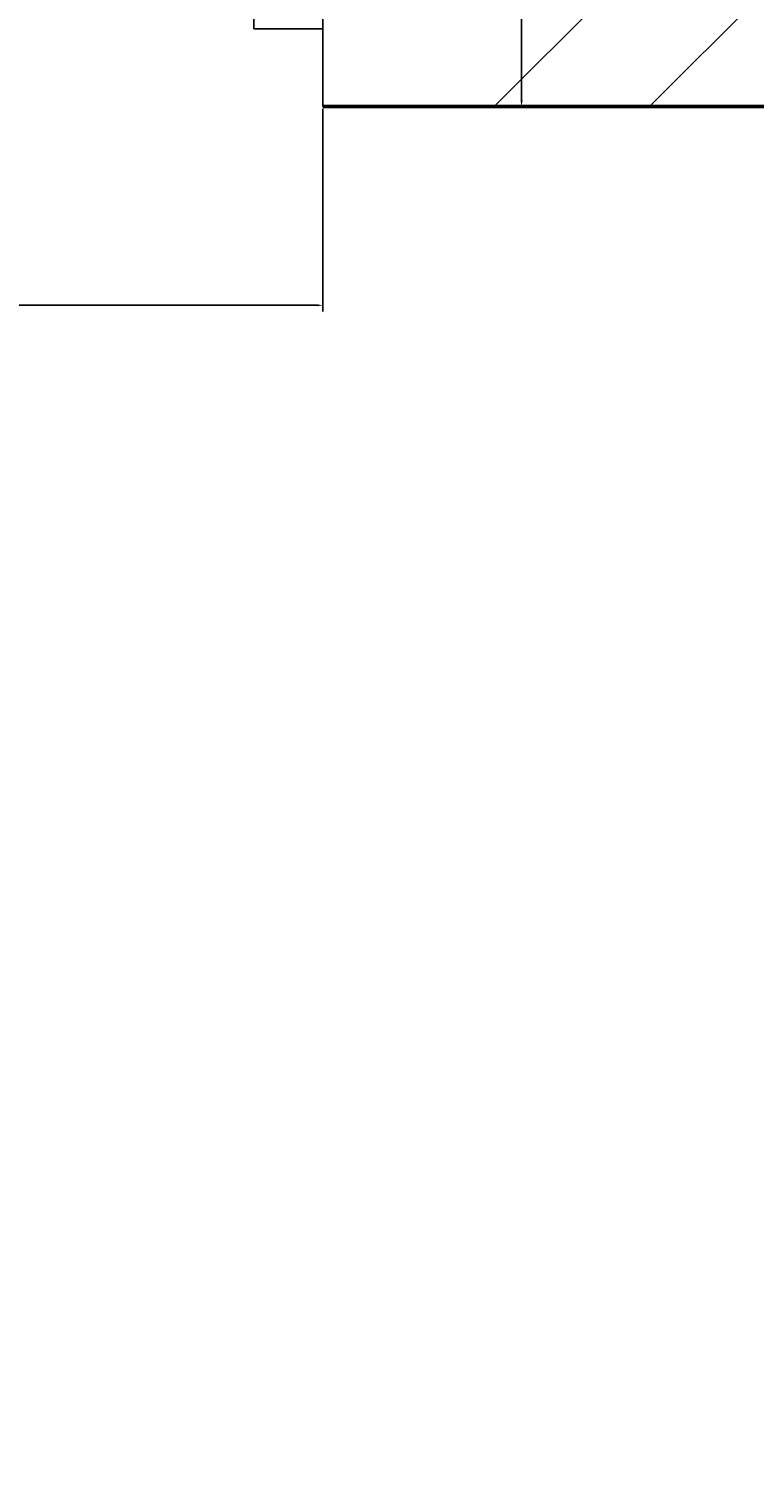
# Model space of a CAD drawing. Units: inches. Extents: x 963 to 2075, y 289 to 2657.
# Tile 65 of 98: x 1245 to 1266, y 2284 to 2325. Entities that reach past the tile are written whole.
import ezdxf

# ---------------------------------------------------------------- set-up
doc = ezdxf.new("R2010")
doc.units = ezdxf.units.IN
for name, color, linetype, lineweight in [('A-ANNO-DIMS', 2, 'Continuous', 18), ('A-DOOR', 4, 'Continuous', 25), ('A-WALL', 7, 'Continuous', 50), ('A-WALL-PATT', 8, 'Continuous', 13)]:
    doc.layers.add(name, color=color, linetype=linetype, lineweight=lineweight)
doc.styles.get("Standard").update_dxf_attribs({"font": 'arial.ttf'})
doc.dimstyles.get("Standard").update_dxf_attribs({"dimtxt": 0.18, "dimasz": 0.18, "dimexe": 0.18, "dimexo": 0.0625, "dimgap": 0.09, "dimtad": 0, "dimtih": 1, "dimtoh": 1, "dimdec": 4, "dimzin": 0, "dimdsep": 46, "dimtxsty": 'Standard', "dimcen": 0.09, "dimadec": 0, "dimazin": 0, "dimtfac": 1, "dimtdec": 4, "dimtofl": 0, "dimtmove": 0, "dimatfit": 3, "dimfxl": 1, "dimtolj": 1, "dimtzin": 0, "dimarcsym": 0})

# ---------------------------------------------------------------- blocks, each defined once
blk = doc.blocks.new('DOOR-1')
for p, q in [((25.385, 2.25), (25.385, 38.25)), ((0.325, 4.5), (0.325, 0)), ((27.385, 4.5), (27.385, 0)), ((0.325, 0), (0.325, 2.25)), ((0.325, 2.25), (2.325, 2.25)), ((27.385, 2.25), (25.385, 2.25)), ((27.385, 0), (27.385, 2.25))]:
    blk.add_line(p, q)
blk.add_arc((25.385, 12.864), 25.386, 90, 204.7158)
blk = doc.blocks.new('*D30')
at = {"layer": 'A-ANNO-DIMS', "color": 0, "lineweight": -2, "transparency": 16777216}
for p, q in [((1253.776, 2361.068), (1259.631, 2361.068)), ((1259.451, 2360.888), (1259.451, 2342.126)), ((1259.451, 2322.998), (1259.451, 2341.759)), ((1253.776, 2322.818), (1259.631, 2322.818))]:
    blk.add_line(p, q, dxfattribs=at)
at = {"layer": 'A-ANNO-DIMS', "color": 0, "transparency": 16777216}
for points in [[(1259.421, 2360.888), (1259.481, 2360.888), (1259.451, 2361.068)], [(1259.421, 2322.998), (1259.481, 2322.998), (1259.451, 2322.818)]]:
    blk.add_solid(points, dxfattribs=at)
at = {"layer": 'Defpoints', "color": 0, "transparency": 16777216}
for p in [(1253.714, 2361.068), (1259.451, 2361.068), (1253.714, 2322.818)]:
    blk.add_point(p, dxfattribs=at)
at = {"layer": 'A-ANNO-DIMS', "color": 0, "transparency": 16777216, "insert": (1259.451, 2341.943), "char_height": 0.18, "attachment_point": 5}
blk.add_mtext('\\A1;DOOR D1 38 TYP.', dxfattribs=at)
blk = doc.blocks.new('*D31')
at = {"layer": 'A-ANNO-DIMS', "color": 0, "lineweight": -2, "transparency": 16777216}
for p, q in [((1225.036, 2322.755), (1225.036, 2316.9)), ((1253.714, 2322.755), (1253.714, 2316.9)), ((1225.216, 2317.08), (1238.845, 2317.08)), ((1253.534, 2317.08), (1239.904, 2317.08))]:
    blk.add_line(p, q, dxfattribs=at)
at = {"layer": 'A-ANNO-DIMS', "color": 0, "transparency": 16777216}
for points in [[(1225.216, 2317.11), (1225.216, 2317.05), (1225.036, 2317.08)], [(1253.534, 2317.11), (1253.534, 2317.05), (1253.714, 2317.08)]]:
    blk.add_solid(points, dxfattribs=at)
at = {"layer": 'Defpoints', "color": 0, "transparency": 16777216}
for p in [(1225.036, 2322.818), (1253.714, 2322.818), (1253.714, 2317.08)]:
    blk.add_point(p, dxfattribs=at)
at = {"layer": 'A-ANNO-DIMS', "color": 0, "transparency": 16777216, "insert": (1239.375, 2317.08), "char_height": 0.18, "attachment_point": 5}
blk.add_mtext('\\A1;29 TYP.', dxfattribs=at)

msp = doc.modelspace()

# ---------------------------------------------------------------- hatches: boundary and pattern name
at = {"layer": 'A-WALL-PATT'}
h = msp.add_hatch(dxfattribs=at)
h.set_pattern_fill('ANSI32', color=256)
h.paths.add_polyline_path([(1296.922, 2558.318), (1203.922, 2558.318), (1203.922, 2493.818), (1191.533, 2493.818), (1191.533, 2489.318), (1211.063, 2489.318), (1211.063, 2492.02), (1211.063, 2493.818), (1208.422, 2493.818), (1208.422, 2553.818), (1292.422, 2553.818), (1292.422, 2538.863), (1296.922, 2538.863)])
h.paths.add_polyline_path([(1442.422, 2558.318), (1349.422, 2558.318), (1349.422, 2538.943), (1353.922, 2538.943), (1353.922, 2553.818), (1437.922, 2553.818), (1437.922, 2493.818), (1434.542, 2493.818), (1434.542, 2489.318), (1448.311, 2489.318), (1448.311, 2491.568), (1448.311, 2493.818), (1442.422, 2493.818)])
h.paths.add_polyline_path([(1415.554, 2491.568), (1415.554, 2493.818), (1340.941, 2493.818), (1340.941, 2489.318), (1371.922, 2489.318), (1371.922, 2378.318), (1367.596, 2378.318), (1367.596, 2373.818), (1371.922, 2373.818), (1371.922, 2355.185), (1376.422, 2355.185), (1376.422, 2489.318), (1415.554, 2489.318)])
h.paths.add_polyline_path([(1304.941, 2491.568), (1304.941, 2493.818), (1296.922, 2493.818), (1296.922, 2514.863), (1292.422, 2514.863), (1292.422, 2493.818), (1232.808, 2493.818), (1232.808, 2489.318), (1256.422, 2489.318), (1256.422, 2327.318), (1253.714, 2327.318), (1253.714, 2322.818), (1328.422, 2322.818), (1328.422, 2331.147), (1323.922, 2331.147), (1323.922, 2327.318), (1260.922, 2327.318), (1260.922, 2373.818), (1323.922, 2373.818), (1323.922, 2357.812), (1328.422, 2357.812), (1328.422, 2373.818), (1346.007, 2373.818), (1346.007, 2376.068), (1346.007, 2378.318), (1260.922, 2378.318), (1260.922, 2489.318), (1304.941, 2489.318)])
h.paths.add_polyline_path([(1226.654, 2327.318), (1124.422, 2327.318), (1124.422, 2347.447), (1119.922, 2347.447), (1119.922, 2322.818), (1163.422, 2322.818), (1163.422, 2305.435), (1165.672, 2305.435), (1167.922, 2305.435), (1167.922, 2322.818), (1226.654, 2322.818), (1226.654, 2325.068)])
h.paths.add_polyline_path([(1095.922, 2489.318), (1124.422, 2489.318), (1131.533, 2489.318), (1131.533, 2491.568), (1131.533, 2493.818), (1119.922, 2493.818), (1091.422, 2493.818), (1091.422, 2417.318), (1095.922, 2417.318), (1119.922, 2417.318), (1119.922, 2407.447), (1124.422, 2407.447), (1124.422, 2421.818), (1095.922, 2421.818)])
h.paths.add_polyline_path([(1512.922, 2558.318), (1508.422, 2558.318), (1508.422, 2493.818), (1503.401, 2493.818), (1503.401, 2489.318), (1508.422, 2489.318), (1508.422, 2327.318), (1376.422, 2327.318), (1376.422, 2330.273), (1371.922, 2330.273), (1371.922, 2298.744), (1376.422, 2298.744), (1376.422, 2322.818), (1508.422, 2322.818), (1508.422, 2165.318), (1504.255, 2165.318), (1504.255, 2160.818), (1508.422, 2160.818), (1508.422, 2108.318), (1512.922, 2108.318), (1512.922, 2160.818), (1516.182, 2160.818), (1516.182, 2163.068), (1516.182, 2165.318), (1512.922, 2165.318), (1512.922, 2322.818), (1644.922, 2322.818), (1644.922, 2298.744), (1649.422, 2298.744), (1649.422, 2322.818), (1649.422, 2330.944), (1647.172, 2330.944), (1644.922, 2330.944), (1644.922, 2327.318), (1512.922, 2327.318), (1512.922, 2489.318), (1516.759, 2489.318), (1516.759, 2491.568), (1516.759, 2493.818), (1512.922, 2493.818)])
h.paths.add_polyline_path([(1671.922, 2558.318), (1578.922, 2558.318), (1578.922, 2493.818), (1573.526, 2493.818), (1573.526, 2489.318), (1586.537, 2489.318), (1586.537, 2491.568), (1586.537, 2493.818), (1583.422, 2493.818), (1583.422, 2553.818), (1667.422, 2553.818), (1667.422, 2541.109), (1671.922, 2541.109)])
h.paths.add_polyline_path([(1681.257, 2493.818), (1671.922, 2493.818), (1671.922, 2517.109), (1667.422, 2517.109), (1667.422, 2493.818), (1610.218, 2493.818), (1610.218, 2489.318), (1644.922, 2489.318), (1644.922, 2357.865), (1649.422, 2357.865), (1649.422, 2373.818), (1652.203, 2373.818), (1652.203, 2375.827), (1652.203, 2378.318), (1649.422, 2378.318), (1649.422, 2489.318), (1681.257, 2489.318), (1681.257, 2491.568)])
h.paths.add_polyline_path([(1821.922, 2558.318), (1728.922, 2558.318), (1728.922, 2541), (1733.422, 2541), (1733.422, 2553.818), (1817.422, 2553.818), (1817.422, 2493.818), (1813.507, 2493.818), (1813.507, 2489.318), (1830.078, 2489.318), (1830.078, 2491.568), (1830.078, 2493.818), (1821.922, 2493.818)])
h.paths.add_polyline_path([(1794.244, 2493.818), (1717.257, 2493.818), (1717.257, 2489.318), (1760.422, 2489.318), (1760.422, 2378.318), (1674.401, 2378.318), (1674.401, 2373.818), (1692.922, 2373.818), (1692.922, 2356.954), (1697.422, 2356.954), (1697.422, 2373.818), (1760.422, 2373.818), (1760.422, 2327.318), (1697.422, 2327.318), (1697.422, 2333.341), (1692.922, 2333.341), (1692.922, 2322.818), (1768.037, 2322.818), (1768.037, 2325.068), (1768.037, 2327.318), (1764.922, 2327.318), (1764.922, 2489.318), (1794.244, 2489.318)])
h.paths.add_polyline_path([(1733.422, 2517), (1728.922, 2517), (1728.922, 2493.818), (1733.422, 2493.818)], flags=17)
h.paths.add_polyline_path([(1929.922, 2493.818), (1890.078, 2493.818), (1890.078, 2489.318), (1896.922, 2489.318), (1925.422, 2489.318), (1925.422, 2421.818), (1896.922, 2421.818), (1896.922, 2408.318), (1901.422, 2408.318), (1901.422, 2417.318), (1925.422, 2417.318), (1929.922, 2417.318)])
h.paths.add_polyline_path([(1901.422, 2348.318), (1896.922, 2348.318), (1896.922, 2327.318), (1800.423, 2327.318), (1800.423, 2322.818), (1853.422, 2322.818), (1853.422, 2309.453), (1857.922, 2309.453), (1857.922, 2322.818), (1901.422, 2322.818)])
h.paths.add_polyline_path([(1857.922, 2249.453), (1853.422, 2249.453), (1853.422, 2214.818), (1686.309, 2214.818), (1686.309, 2210.318), (1853.422, 2210.318), (1853.422, 2202.134), (1857.922, 2202.134), (1857.922, 2210.318)])
h.paths.add_polyline_path([(1857.922, 2142.134), (1853.422, 2142.134), (1853.422, 2115.422), (1841.422, 2115.422), (1841.422, 2088.531), (1841.422, 2046.949), (1845.922, 2046.949), (1845.922, 2110.922), (1905.922, 2110.922), (1905.922, 2092.517), (1910.422, 2092.517), (1910.422, 2115.422), (1857.922, 2115.422)])
h.paths.add_polyline_path([(1532.436, 1482.342), (1573.456, 1482.342), (1573.456, 1501), (1532.436, 1501)], flags=9)
h.paths.add_polyline_path([(1438.658, 1486.302), (1479.678, 1486.302), (1479.678, 1504.96), (1438.658, 1504.96)], flags=9)
h.paths.add_polyline_path([(1411.215, 1365.308), (1659.139, 1365.308), (1659.139, 1402.401), (1411.215, 1402.401)], flags=9)
h.paths.add_polyline_path([(1185.671, 2296.298), (1248.16, 2296.298), (1248.16, 2314.955), (1185.671, 2314.955)], flags=9)
h.paths.add_polyline_path([(1177.31, 2187.35), (1216.15, 2187.35), (1216.15, 2206.007), (1177.31, 2206.007)], flags=9)
h.paths.add_polyline_path([(1295.101, 1602.083), (1328.26, 1602.083), (1328.26, 1620.741), (1295.101, 1620.741)], flags=9)
h.paths.add_polyline_path([(1525.126, 2005.99), (1558.39, 2005.99), (1558.39, 2024.648), (1525.126, 2024.648)], flags=9)
h.paths.add_polyline_path([(1459.606, 1977.125), (1472.195, 1977.125), (1472.195, 1987.429), (1459.606, 1987.429)], flags=9)
h.paths.add_polyline_path([(1467.815, 2053.676), (1480.018, 2053.676), (1480.018, 2063.979), (1467.815, 2063.979)], flags=9)
h.paths.add_polyline_path([(1555.184, 2119.02), (1584.563, 2119.02), (1584.563, 2137.678), (1555.184, 2137.678)], flags=25)
h.paths.add_polyline_path([(1405.389, 2115.291), (1444.478, 2115.291), (1444.478, 2133.948), (1405.389, 2133.948)], flags=25)
h.paths.add_polyline_path([(1698.482, 2004.259), (1727.695, 2004.259), (1727.695, 2022.916), (1698.482, 2022.916)], flags=9)
h.paths.add_polyline_path([(1612.158, 1972.855), (1629.016, 1972.855), (1629.016, 1983.159), (1612.158, 1983.159)], flags=9)
h.paths.add_polyline_path([(1608.289, 2060.036), (1625.147, 2060.036), (1625.147, 2070.34), (1608.289, 2070.34)], flags=9)
h.paths.add_polyline_path([(1527.954, 1684.402), (1566.795, 1684.402), (1566.795, 1703.06), (1527.954, 1703.06)], flags=9)
h.paths.add_polyline_path([(1422.792, 1683.59), (1461.633, 1683.59), (1461.633, 1702.247), (1422.792, 1702.247)], flags=9)
h.paths.add_polyline_path([(1531.262, 1732.459), (1574.015, 1732.459), (1574.015, 1751.116), (1531.262, 1751.116)], flags=9)
h.paths.add_polyline_path([(1402.872, 1732.845), (1439.799, 1732.845), (1439.799, 1751.502), (1402.872, 1751.502)], flags=9)
h.paths.add_polyline_path([(1243.122, 1923.132), (1281.962, 1923.132), (1281.962, 1941.79), (1243.122, 1941.79)], flags=9)
h.paths.add_polyline_path([(1181.752, 1792.268), (1244.241, 1792.268), (1244.241, 1810.926), (1181.752, 1810.926)], flags=9)
h.paths.add_polyline_path([(1265.822, 1670.3), (1316.071, 1670.3), (1316.071, 1688.957), (1265.822, 1688.957)], flags=9)
h.paths.add_polyline_path([(1140.263, 1676.054), (1179.104, 1676.054), (1179.104, 1694.711), (1140.263, 1694.711)], flags=9)
h.paths.add_polyline_path([(1107.49, 1490.889), (1143.374, 1490.889), (1143.374, 1509.546), (1107.49, 1509.546)], flags=9)
h.paths.add_polyline_path([(1217.584, 1483.899), (1246.741, 1483.899), (1246.741, 1502.556), (1217.584, 1502.556)], flags=9)
h.paths.add_polyline_path([(1389.21, 1486.919), (1418.367, 1486.919), (1418.367, 1505.576), (1389.21, 1505.576)], flags=9)
h.paths.add_polyline_path([(1672.208, 1602.083), (1705.366, 1602.083), (1705.366, 1620.741), (1672.208, 1620.741)], flags=9)
h.paths.add_polyline_path([(1752.082, 1522.638), (1781.24, 1522.638), (1781.24, 1541.295), (1752.082, 1541.295)], flags=9)
h.paths.add_polyline_path([(1848.275, 1491.26), (1884.158, 1491.26), (1884.158, 1509.918), (1848.275, 1509.918)], flags=9)
h.paths.add_polyline_path([(1822.47, 1685.62), (1861.31, 1685.62), (1861.31, 1704.278), (1822.47, 1704.278)], flags=9)
h.paths.add_polyline_path([(1713.195, 1672.232), (1763.444, 1672.232), (1763.444, 1690.889), (1713.195, 1690.889)], flags=9)
h.paths.add_polyline_path([(1736.619, 1790.578), (1799.109, 1790.578), (1799.109, 1809.235), (1736.619, 1809.235)], flags=9)
h.paths.add_polyline_path([(1691.491, 1916.355), (1730.332, 1916.355), (1730.332, 1935.013), (1691.491, 1935.013)], flags=9)
h.paths.add_polyline_path([(1764.872, 1973.922), (1794.306, 1973.922), (1794.306, 1992.58), (1764.872, 1992.58)], flags=9)
h.paths.add_polyline_path([(1767.854, 2034.017), (1797.288, 2034.017), (1797.288, 2052.674), (1767.854, 2052.674)], flags=9)
h.paths.add_polyline_path([(1851.593, 2060.331), (1880.751, 2060.331), (1880.751, 2078.989), (1851.593, 2078.989)], flags=25)
h.paths.add_polyline_path([(1688.491, 2086.874), (1727.332, 2086.874), (1727.332, 2105.531), (1688.491, 2105.531)], flags=9)
h.paths.add_polyline_path([(1537.743, 2293.581), (1580.495, 2293.581), (1580.495, 2312.239), (1537.743, 2312.239)], flags=25)
h.paths.add_polyline_path([(1425.587, 2296.109), (1468.34, 2296.109), (1468.34, 2314.766), (1425.587, 2314.766)], flags=25)
h.paths.add_polyline_path([(1278.518, 2004.184), (1307.72, 2004.184), (1307.72, 2022.841), (1278.518, 2022.841)], flags=9)
h.paths.add_polyline_path([(1193.282, 1973.635), (1222.715, 1973.635), (1222.715, 1992.292), (1193.282, 1992.292)], flags=9)
h.paths.add_polyline_path([(1192.411, 2040.577), (1221.845, 2040.577), (1221.845, 2059.234), (1192.411, 2059.234)], flags=9)
h.paths.add_polyline_path([(1130.603, 1951.393), (1159.76, 1951.393), (1159.76, 1970.05), (1130.603, 1970.05)], flags=9)
h.paths.add_polyline_path([(1132.827, 2052.494), (1161.984, 2052.494), (1161.984, 2071.151), (1132.827, 2071.151)], flags=9)
h.paths.add_polyline_path([(1265.128, 2334.619), (1315.377, 2334.619), (1315.377, 2353.277), (1265.128, 2353.277)], flags=25)
h.paths.add_polyline_path([(1136.741, 2330.785), (1175.582, 2330.785), (1175.582, 2349.443), (1136.741, 2349.443)], flags=9)
h.paths.add_polyline_path([(1287.422, 2417.204), (1320.58, 2417.204), (1320.58, 2435.861), (1287.422, 2435.861)], flags=25)
h.paths.add_polyline_path([(1430.988, 2329.159), (1469.828, 2329.159), (1469.828, 2347.816), (1430.988, 2347.816)], flags=25)
h.paths.add_polyline_path([(1525.424, 2329.213), (1564.264, 2329.213), (1564.264, 2347.87), (1525.424, 2347.87)], flags=25)
h.paths.add_polyline_path([(1684.525, 2382.799), (1717.683, 2382.799), (1717.683, 2401.457), (1684.525, 2401.457)], flags=25)
h.paths.add_polyline_path([(1704.805, 2340.293), (1755.054, 2340.293), (1755.054, 2358.95), (1704.805, 2358.95)], flags=25)
h.paths.add_polyline_path([(1694.113, 2287.757), (1756.602, 2287.757), (1756.602, 2306.414), (1694.113, 2306.414)], flags=9)
h.paths.add_polyline_path([(1815.778, 2329.861), (1854.618, 2329.861), (1854.618, 2348.518), (1815.778, 2348.518)], flags=9)
h.paths.add_polyline_path([(1842.873, 2514.256), (1878.756, 2514.256), (1878.756, 2532.914), (1842.873, 2532.914)], flags=9)
h.paths.add_polyline_path([(1769.513, 2531.447), (1798.671, 2531.447), (1798.671, 2550.104), (1769.513, 2550.104)], flags=25)
h.paths.add_polyline_path([(1594.772, 2518.468), (1623.93, 2518.468), (1623.93, 2537.125), (1594.772, 2537.125)], flags=25)
h.paths.add_polyline_path([(1520.723, 2516.185), (1556.606, 2516.185), (1556.606, 2534.842), (1520.723, 2534.842)], flags=25)
h.paths.add_polyline_path([(1464.456, 2516.694), (1500.34, 2516.694), (1500.34, 2535.351), (1464.456, 2535.351)], flags=25)
h.paths.add_polyline_path([(1365.696, 2528.97), (1394.854, 2528.97), (1394.854, 2547.627), (1365.696, 2547.627)], flags=25)
h.paths.add_polyline_path([(1222.838, 2516.231), (1251.995, 2516.231), (1251.995, 2534.889), (1222.838, 2534.889)], flags=25)
h.paths.add_polyline_path([(1104.545, 2509.6), (1140.429, 2509.6), (1140.429, 2528.257), (1104.545, 2528.257)], flags=9)
h = msp.add_hatch(dxfattribs=at)
h.set_pattern_fill('ANSI32', color=256)
h.paths.add_polyline_path([(1335.968, 2212.568), (1335.968, 2214.818), (1167.922, 2214.818), (1167.922, 2245.435), (1163.422, 2245.435), (1163.422, 2210.318), (1163.422, 2194.812), (1167.922, 2194.812), (1167.922, 2210.318), (1335.968, 2210.318)])
h.paths.add_polyline_path([(1532.436, 1482.342), (1573.456, 1482.342), (1573.456, 1501), (1532.436, 1501)], flags=9)
h.paths.add_polyline_path([(1438.658, 1486.302), (1479.678, 1486.302), (1479.678, 1504.96), (1438.658, 1504.96)], flags=9)
h.paths.add_polyline_path([(1411.215, 1365.308), (1659.139, 1365.308), (1659.139, 1402.401), (1411.215, 1402.401)], flags=9)
h.paths.add_polyline_path([(1185.671, 2296.298), (1248.16, 2296.298), (1248.16, 2314.955), (1185.671, 2314.955)], flags=9)
h.paths.add_polyline_path([(1177.31, 2187.35), (1216.15, 2187.35), (1216.15, 2206.007), (1177.31, 2206.007)], flags=9)
h.paths.add_polyline_path([(1295.101, 1602.083), (1328.26, 1602.083), (1328.26, 1620.741), (1295.101, 1620.741)], flags=9)
h.paths.add_polyline_path([(1525.126, 2005.99), (1558.39, 2005.99), (1558.39, 2024.648), (1525.126, 2024.648)], flags=9)
h.paths.add_polyline_path([(1459.606, 1977.125), (1472.195, 1977.125), (1472.195, 1987.429), (1459.606, 1987.429)], flags=9)
h.paths.add_polyline_path([(1467.815, 2053.676), (1480.018, 2053.676), (1480.018, 2063.979), (1467.815, 2063.979)], flags=9)
h.paths.add_polyline_path([(1555.184, 2119.02), (1584.563, 2119.02), (1584.563, 2137.678), (1555.184, 2137.678)], flags=9)
h.paths.add_polyline_path([(1405.389, 2115.291), (1444.478, 2115.291), (1444.478, 2133.948), (1405.389, 2133.948)], flags=9)
h.paths.add_polyline_path([(1698.482, 2004.259), (1727.695, 2004.259), (1727.695, 2022.916), (1698.482, 2022.916)], flags=9)
h.paths.add_polyline_path([(1612.158, 1972.855), (1629.016, 1972.855), (1629.016, 1983.159), (1612.158, 1983.159)], flags=9)
h.paths.add_polyline_path([(1608.289, 2060.036), (1625.147, 2060.036), (1625.147, 2070.34), (1608.289, 2070.34)], flags=9)
h.paths.add_polyline_path([(1527.954, 1684.402), (1566.795, 1684.402), (1566.795, 1703.06), (1527.954, 1703.06)], flags=9)
h.paths.add_polyline_path([(1422.792, 1683.59), (1461.633, 1683.59), (1461.633, 1702.247), (1422.792, 1702.247)], flags=9)
h.paths.add_polyline_path([(1531.262, 1732.459), (1574.015, 1732.459), (1574.015, 1751.116), (1531.262, 1751.116)], flags=9)
h.paths.add_polyline_path([(1402.872, 1732.845), (1439.799, 1732.845), (1439.799, 1751.502), (1402.872, 1751.502)], flags=9)
h.paths.add_polyline_path([(1243.122, 1923.132), (1281.962, 1923.132), (1281.962, 1941.79), (1243.122, 1941.79)], flags=9)
h.paths.add_polyline_path([(1181.752, 1792.268), (1244.241, 1792.268), (1244.241, 1810.926), (1181.752, 1810.926)], flags=9)
h.paths.add_polyline_path([(1265.822, 1670.3), (1316.071, 1670.3), (1316.071, 1688.957), (1265.822, 1688.957)], flags=9)
h.paths.add_polyline_path([(1140.263, 1676.054), (1179.104, 1676.054), (1179.104, 1694.711), (1140.263, 1694.711)], flags=9)
h.paths.add_polyline_path([(1107.49, 1490.889), (1143.374, 1490.889), (1143.374, 1509.546), (1107.49, 1509.546)], flags=9)
h.paths.add_polyline_path([(1217.584, 1483.899), (1246.741, 1483.899), (1246.741, 1502.556), (1217.584, 1502.556)], flags=9)
h.paths.add_polyline_path([(1389.21, 1486.919), (1418.367, 1486.919), (1418.367, 1505.576), (1389.21, 1505.576)], flags=9)
h.paths.add_polyline_path([(1672.208, 1602.083), (1705.366, 1602.083), (1705.366, 1620.741), (1672.208, 1620.741)], flags=9)
h.paths.add_polyline_path([(1752.082, 1522.638), (1781.24, 1522.638), (1781.24, 1541.295), (1752.082, 1541.295)], flags=9)
h.paths.add_polyline_path([(1848.275, 1491.26), (1884.158, 1491.26), (1884.158, 1509.918), (1848.275, 1509.918)], flags=9)
h.paths.add_polyline_path([(1822.47, 1685.62), (1861.31, 1685.62), (1861.31, 1704.278), (1822.47, 1704.278)], flags=9)
h.paths.add_polyline_path([(1713.195, 1672.232), (1763.444, 1672.232), (1763.444, 1690.889), (1713.195, 1690.889)], flags=9)
h.paths.add_polyline_path([(1736.619, 1790.578), (1799.109, 1790.578), (1799.109, 1809.235), (1736.619, 1809.235)], flags=9)
h.paths.add_polyline_path([(1691.491, 1916.355), (1730.332, 1916.355), (1730.332, 1935.013), (1691.491, 1935.013)], flags=9)
h.paths.add_polyline_path([(1764.872, 1973.922), (1794.306, 1973.922), (1794.306, 1992.58), (1764.872, 1992.58)], flags=9)
h.paths.add_polyline_path([(1767.854, 2034.017), (1797.288, 2034.017), (1797.288, 2052.674), (1767.854, 2052.674)], flags=9)
h.paths.add_polyline_path([(1851.593, 2060.331), (1880.751, 2060.331), (1880.751, 2078.989), (1851.593, 2078.989)], flags=9)
h.paths.add_polyline_path([(1688.491, 2086.874), (1727.332, 2086.874), (1727.332, 2105.531), (1688.491, 2105.531)], flags=9)
h.paths.add_polyline_path([(1537.743, 2293.581), (1580.495, 2293.581), (1580.495, 2312.239), (1537.743, 2312.239)], flags=9)
h.paths.add_polyline_path([(1425.587, 2296.109), (1468.34, 2296.109), (1468.34, 2314.766), (1425.587, 2314.766)], flags=9)
h.paths.add_polyline_path([(1278.518, 2004.184), (1307.72, 2004.184), (1307.72, 2022.841), (1278.518, 2022.841)], flags=9)
h.paths.add_polyline_path([(1193.282, 1973.635), (1222.715, 1973.635), (1222.715, 1992.292), (1193.282, 1992.292)], flags=9)
h.paths.add_polyline_path([(1192.411, 2040.577), (1221.845, 2040.577), (1221.845, 2059.234), (1192.411, 2059.234)], flags=9)
h.paths.add_polyline_path([(1130.603, 1951.393), (1159.76, 1951.393), (1159.76, 1970.05), (1130.603, 1970.05)], flags=9)
h.paths.add_polyline_path([(1132.827, 2052.494), (1161.984, 2052.494), (1161.984, 2071.151), (1132.827, 2071.151)], flags=9)
h.paths.add_polyline_path([(1265.128, 2334.619), (1315.377, 2334.619), (1315.377, 2353.277), (1265.128, 2353.277)], flags=9)
h.paths.add_polyline_path([(1136.741, 2330.785), (1175.582, 2330.785), (1175.582, 2349.443), (1136.741, 2349.443)], flags=9)
h.paths.add_polyline_path([(1287.422, 2417.204), (1320.58, 2417.204), (1320.58, 2435.861), (1287.422, 2435.861)], flags=9)
h.paths.add_polyline_path([(1430.988, 2329.159), (1469.828, 2329.159), (1469.828, 2347.816), (1430.988, 2347.816)], flags=9)
h.paths.add_polyline_path([(1525.424, 2329.213), (1564.264, 2329.213), (1564.264, 2347.87), (1525.424, 2347.87)], flags=9)
h.paths.add_polyline_path([(1684.525, 2382.799), (1717.683, 2382.799), (1717.683, 2401.457), (1684.525, 2401.457)], flags=9)
h.paths.add_polyline_path([(1704.805, 2340.293), (1755.054, 2340.293), (1755.054, 2358.95), (1704.805, 2358.95)], flags=9)
h.paths.add_polyline_path([(1694.113, 2287.757), (1756.602, 2287.757), (1756.602, 2306.414), (1694.113, 2306.414)], flags=9)
h.paths.add_polyline_path([(1815.778, 2329.861), (1854.618, 2329.861), (1854.618, 2348.518), (1815.778, 2348.518)], flags=9)
h.paths.add_polyline_path([(1842.873, 2514.256), (1878.756, 2514.256), (1878.756, 2532.914), (1842.873, 2532.914)], flags=9)
h.paths.add_polyline_path([(1769.513, 2531.447), (1798.671, 2531.447), (1798.671, 2550.104), (1769.513, 2550.104)], flags=9)
h.paths.add_polyline_path([(1594.772, 2518.468), (1623.93, 2518.468), (1623.93, 2537.125), (1594.772, 2537.125)], flags=9)
h.paths.add_polyline_path([(1520.723, 2516.185), (1556.606, 2516.185), (1556.606, 2534.842), (1520.723, 2534.842)], flags=9)
h.paths.add_polyline_path([(1464.456, 2516.694), (1500.34, 2516.694), (1500.34, 2535.351), (1464.456, 2535.351)], flags=9)
h.paths.add_polyline_path([(1365.696, 2528.97), (1394.854, 2528.97), (1394.854, 2547.627), (1365.696, 2547.627)], flags=9)
h.paths.add_polyline_path([(1222.838, 2516.231), (1251.995, 2516.231), (1251.995, 2534.889), (1222.838, 2534.889)], flags=9)
h.paths.add_polyline_path([(1104.545, 2509.6), (1140.429, 2509.6), (1140.429, 2528.257), (1104.545, 2528.257)], flags=9)

# ---------------------------------------------------------------- linework, layer by layer
at = {"layer": 'A-WALL'}
msp.add_line((1253.714, 2322.818), (1328.422, 2322.818), dxfattribs=at)

# ---------------------------------------------------------------- block references
at = {"layer": 'A-DOOR'}
msp.add_blockref('DOOR-1', (1226.329, 2322.818), dxfattribs=at)

# ---------------------------------------------------------------- dimensions: what is measured, and where the dimension line sits
at = {"layer": 'A-ANNO-DIMS'}
dim = msp.add_linear_dim(base=(1259.451, 2361.068), p1=(1253.714, 2322.818), p2=(1253.714, 2361.068), angle=90, text='DOOR D1 <> TYP.', dimstyle='Standard', override={"dimdec": 0, "dimlfac": 1, "dimrnd": 0, "dimzin": 0, "dimdsep": 46, "dimlunit": 2}, dxfattribs=at)
dim.commit()
dim.dimension.update_dxf_attribs({"geometry": '*D30', "text_midpoint": (1259.451, 2341.943)})
dim = msp.add_linear_dim(base=(1253.714, 2317.08), p1=(1225.036, 2322.818), p2=(1253.714, 2322.818), text='<> TYP.', dimstyle='Standard', override={"dimdec": 0, "dimlfac": 1, "dimrnd": 0, "dimzin": 0, "dimdsep": 46, "dimlunit": 2}, dxfattribs=at)
dim.commit()
dim.dimension.update_dxf_attribs({"geometry": '*D31', "text_midpoint": (1239.375, 2317.08)})

doc.saveas('drawing.dxf')
